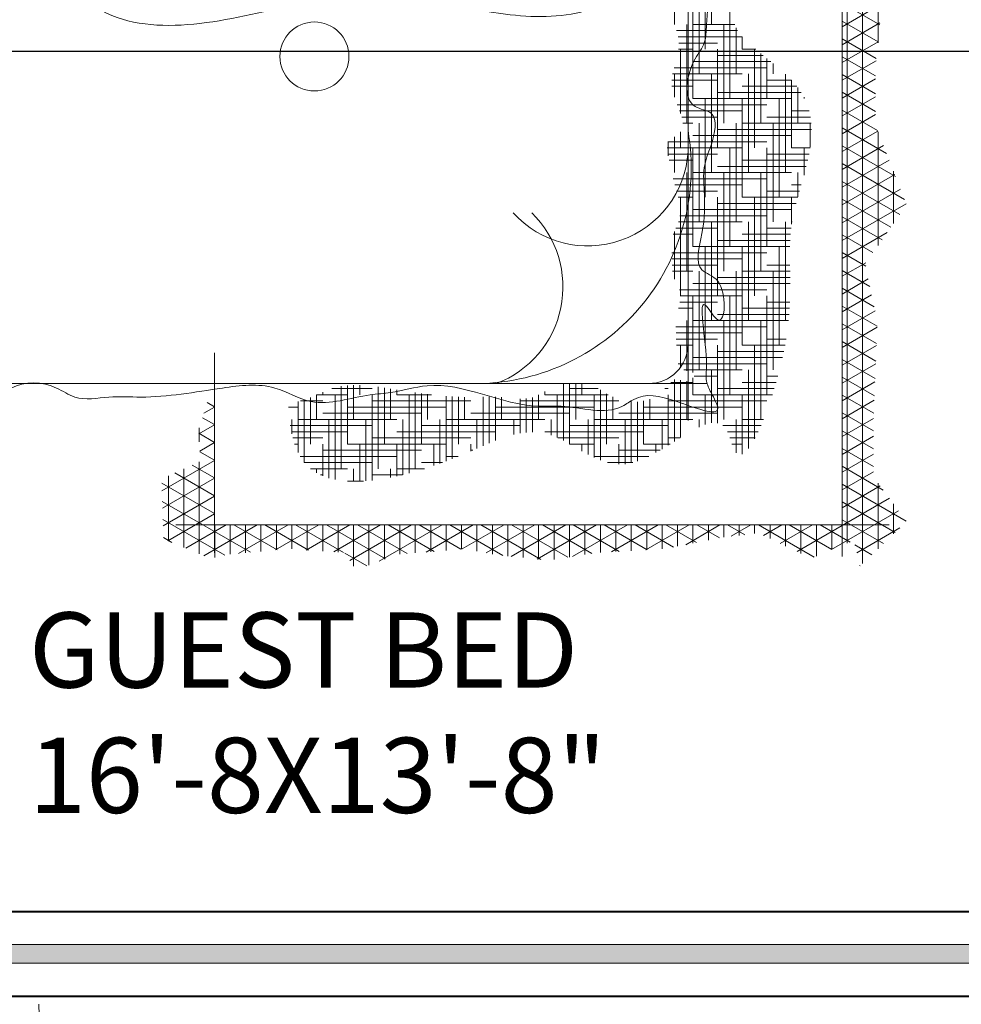
# Model space of a CAD drawing. Units: inches. Extents: x 2330 to 3943, y 1763 to 3461.
# Tile 4 of 40: x 2533 to 2634, y 2211 to 2316. Entities that reach past the tile are written whole.
import ezdxf

# ---------------------------------------------------------------- set-up
doc = ezdxf.new("R2010")
doc.units = ezdxf.units.IN
for name, color, linetype, lineweight in [('A-ANNO-DIMS', 2, 'Continuous', 18), ('A-AREA-IDEN', 7, 'Continuous', 18), ('A-FURN', 8, 'Continuous', 13), ('A-GLAZ', 4, 'Continuous', 18), ('A-WALL', 7, 'Continuous', 40), ('L-PLNT', 94, 'Continuous', 13)]:
    doc.layers.add(name, color=color, linetype=linetype, lineweight=lineweight)
doc.styles.get("Standard").update_dxf_attribs({"font": 'arial.ttf'})
doc.dimstyles.get("Standard").update_dxf_attribs({"dimtxt": 0.18, "dimasz": 0.18, "dimexe": 0.18, "dimexo": 0.0625, "dimgap": 0.09, "dimtad": 0, "dimtih": 1, "dimtoh": 1, "dimdec": 4, "dimzin": 0, "dimdsep": 46, "dimtxsty": 'Standard', "dimcen": 0.09, "dimadec": 0, "dimazin": 0, "dimtfac": 1, "dimtdec": 4, "dimtofl": 0, "dimtmove": 0, "dimatfit": 3, "dimfxl": 1, "dimtolj": 1, "dimtzin": 0, "dimarcsym": 0})

# ---------------------------------------------------------------- blocks, each defined once
blk = doc.blocks.new('A$C200C7901')
for p, q in [((2.3121, 1.6596), (2.3121, 0.0201)), ((2, 0.2957), (2, 1.2957)), ((2.0224, 0.9977), (2.0224, 1.1977)), ((2.0224, 0.9977), (2.0224, 1.1977)), ((1.9974, 0.5977), (1.9974, 0.7977)), ((1.9974, 0.5977), (1.9974, 0.7977)), ((2.0724, 0.5977), (2.0724, 0.7977)), ((2.0724, 0.5977), (2.0724, 0.7977)), ((2.1474, 0.5977), (2.1474, 0.7977)), ((2.1474, 0.5977), (2.1474, 0.7977)), ((1.9849, 0.5477), (1.9849, 0.7477)), ((1.9849, 0.5477), (1.9849, 0.7477)), ((2.0599, 0.5477), (2.0599, 0.7477)), ((2.0599, 0.5477), (2.0599, 0.7477)), ((2.1349, 0.5477), (2.1349, 0.7477)), ((2.1349, 0.5477), (2.1349, 0.7477)), ((1.0407, 0.0275), (1.0407, 0.4323)), ((0.4061, 0.3703), (2.0386, 0.3703)), ((2.4073, 0.0839), (0.9625, 0.0839))]:
    blk.add_line(p, q)
at = {"linetype": 'ByBlock'}
for p, q in [((2.3224, 0.0468), (2.3224, 1.6627)), ((2.3224, 0.0468), (2.3224, 1.6627)), ((2.3537, 0.0056), (2.3537, 1.634)), ((2.3537, 0.0056), (2.3537, 1.634)), ((2.0474, 1.0977), (2.0474, 1.2977)), ((2.0474, 1.0977), (2.0474, 1.2977)), ((2.3849, 1.0607), (2.3849, 1.3013)), ((2.3849, 1.0607), (2.3849, 1.3013)), ((1.9724, 1.0977), (1.9724, 1.2927)), ((1.9724, 1.0977), (1.9724, 1.2927)), ((2.0349, 1.0477), (2.0349, 1.2477)), ((2.0349, 1.0477), (2.0349, 1.2477)), ((2.0099, 0.9477), (2.0099, 1.1477)), ((2.0099, 0.9477), (2.0099, 1.1477)), ((2.0849, 0.9477), (2.0849, 1.1477)), ((2.0849, 0.9477), (2.0849, 1.1477)), ((2.3121, 1.1408), (2.3884, 1.0967)), ((2.3121, 1.1408), (2.3884, 1.0967)), ((2.3121, 1.0928), (2.3915, 1.1386)), ((2.3121, 1.0928), (2.3915, 1.1386)), ((1.9974, 0.8977), (1.9974, 1.0977)), ((1.9974, 0.8977), (1.9974, 1.0977)), ((2.0099, 1.0977), (2.095, 1.0977)), ((2.0099, 1.0977), (2.095, 1.0977)), ((2.0724, 0.8977), (2.0724, 1.0977)), ((2.0724, 0.8977), (2.0724, 1.0977)), ((2.3121, 1.1047), (2.3851, 1.0625)), ((2.3121, 1.1047), (2.3851, 1.0625)), ((2.3121, 1.0567), (2.3887, 1.1009)), ((2.3121, 1.0567), (2.3887, 1.1009)), ((1.9763, 1.0852), (2.1005, 1.0852)), ((1.9763, 1.0852), (2.1005, 1.0852)), ((2.0974, 0.9977), (2.0974, 1.0909)), ((2.0974, 0.9977), (2.0974, 1.0909)), ((1.9799, 1.0727), (2.1099, 1.0727)), ((1.9799, 1.0727), (2.1099, 1.0727)), ((1.9815, 1.0602), (2.0599, 1.0602)), ((1.9815, 1.0602), (2.0599, 1.0602)), ((2.1099, 1.0477), (2.1099, 1.0729)), ((2.1099, 1.0477), (2.1099, 1.0729)), ((2.3121, 1.0686), (2.3813, 1.0286)), ((2.3121, 1.0686), (2.3813, 1.0286)), ((2.3121, 1.0206), (2.3851, 1.0628)), ((2.3121, 1.0206), (2.3851, 1.0628)), ((1.981, 1.0477), (2.0099, 1.0477)), ((1.981, 1.0477), (2.0099, 1.0477)), ((1.9849, 0.9171), (1.9849, 1.0477)), ((1.9849, 0.9171), (1.9849, 1.0477)), ((2.0599, 0.8477), (2.0599, 1.0477)), ((2.0599, 0.8477), (2.0599, 1.0477)), ((2.1099, 1.0477), (2.137, 1.0477)), ((2.1099, 1.0477), (2.137, 1.0477)), ((2.1349, 0.8477), (2.1349, 1.0477)), ((2.1349, 0.8477), (2.1349, 1.0477)), ((2.1474, 0.8977), (2.1474, 1.0391)), ((2.1474, 0.8977), (2.1474, 1.0391)), ((2.0099, 1.0227), (2.1678, 1.0227)), ((2.0099, 1.0227), (2.1678, 1.0227)), ((2.0599, 1.0352), (2.1523, 1.0352)), ((2.0599, 1.0352), (2.1523, 1.0352)), ((2.1599, 0.9477), (2.1599, 1.029)), ((2.1599, 0.9477), (2.1599, 1.029)), ((2.1724, 0.9977), (2.1724, 1.0189)), ((2.1724, 0.9977), (2.1724, 1.0189)), ((2.3121, 1.0325), (2.3795, 0.9936)), ((2.3121, 1.0325), (2.3795, 0.9936)), ((2.3121, 0.9846), (2.3809, 1.0242)), ((2.3121, 0.9846), (2.3809, 1.0242)), ((1.9688, 0.9977), (2.1099, 0.9977)), ((1.9688, 0.9977), (2.1099, 0.9977)), ((1.9718, 1.0102), (2.1599, 1.0102)), ((1.9718, 1.0102), (2.1599, 1.0102)), ((1.9724, 0.9504), (1.9724, 0.9977)), ((1.9724, 0.9504), (1.9724, 0.9977)), ((2.0474, 0.7977), (2.0474, 0.9977)), ((2.0474, 0.7977), (2.0474, 0.9977)), ((2.1224, 0.7977), (2.1224, 0.9977)), ((2.1224, 0.7977), (2.1224, 0.9977)), ((1.9671, 0.9852), (2.0599, 0.9852)), ((1.9671, 0.9852), (2.0599, 0.9852)), ((2.1599, 0.9852), (2.2095, 0.9852)), ((2.1599, 0.9852), (2.2095, 0.9852)), ((2.1974, 0.7977), (2.1974, 0.9972)), ((2.1974, 0.7977), (2.1974, 0.9972)), ((2.2099, 0.8477), (2.2099, 0.9848)), ((2.2099, 0.8477), (2.2099, 0.9848)), ((2.3121, 0.9964), (2.3795, 0.9575)), ((2.3121, 0.9964), (2.3795, 0.9575)), ((2.3121, 0.9485), (2.3795, 0.9874)), ((2.3121, 0.9485), (2.3795, 0.9874)), ((1.9672, 0.9727), (2.0099, 0.9727)), ((1.9672, 0.9727), (2.0099, 0.9727)), ((2.0599, 0.9602), (2.2294, 0.9602)), ((2.0599, 0.9602), (2.2294, 0.9602)), ((2.1099, 0.9727), (2.2204, 0.9727)), ((2.1099, 0.9727), (2.2204, 0.9727)), ((2.2224, 0.8977), (2.2224, 0.9702)), ((2.2224, 0.8977), (2.2224, 0.9702)), ((2.3121, 0.9603), (2.3795, 0.9215)), ((2.3121, 0.9603), (2.3795, 0.9215)), ((2.0099, 0.9477), (2.2099, 0.9477)), ((2.0099, 0.9477), (2.2099, 0.9477)), ((2.0349, 0.7477), (2.0349, 0.9477)), ((2.0349, 0.7477), (2.0349, 0.9477)), ((2.1099, 0.7477), (2.1099, 0.9477)), ((2.1099, 0.7477), (2.1099, 0.9477)), ((2.1849, 0.7477), (2.1849, 0.9477)), ((2.1849, 0.7477), (2.1849, 0.9477)), ((2.2349, 0.9477), (2.2349, 0.9506)), ((2.2349, 0.9477), (2.2349, 0.9506)), ((2.3121, 0.9124), (2.3795, 0.9513)), ((2.3121, 0.9124), (2.3795, 0.9513)), ((1.9781, 0.9352), (2.1599, 0.9352)), ((1.9781, 0.9352), (2.1599, 0.9352)), ((1.9829, 0.9227), (2.1099, 0.9227)), ((1.9829, 0.9227), (2.1099, 0.9227)), ((2.2099, 0.9227), (2.2455, 0.9227)), ((2.2099, 0.9227), (2.2455, 0.9227)), ((2.3121, 0.9243), (2.3838, 0.8829)), ((2.3121, 0.9243), (2.3838, 0.8829)), ((1.9871, 0.9102), (2.0599, 0.9102)), ((1.9871, 0.9102), (2.0599, 0.9102)), ((2.1599, 0.9102), (2.2481, 0.9102)), ((2.1599, 0.9102), (2.2481, 0.9102)), ((2.3121, 0.8763), (2.3795, 0.9152)), ((2.3121, 0.8763), (2.3795, 0.9152)), ((1.9849, 0.8477), (1.9849, 0.88)), ((1.9849, 0.8477), (1.9849, 0.88)), ((1.9894, 0.8977), (2.0099, 0.8977)), ((1.9894, 0.8977), (2.0099, 0.8977)), ((2.0224, 0.6977), (2.0224, 0.8977)), ((2.0224, 0.6977), (2.0224, 0.8977)), ((2.0599, 0.8852), (2.2501, 0.8852)), ((2.0599, 0.8852), (2.2501, 0.8852)), ((2.0974, 0.6977), (2.0974, 0.8977)), ((2.0974, 0.6977), (2.0974, 0.8977)), ((2.1099, 0.8977), (2.2496, 0.8977)), ((2.1099, 0.8977), (2.2496, 0.8977)), ((2.1724, 0.6977), (2.1724, 0.8977)), ((2.1724, 0.6977), (2.1724, 0.8977)), ((2.2474, 0.8489), (2.2474, 0.8977)), ((2.2474, 0.8489), (2.2474, 0.8977)), ((2.3121, 0.8882), (2.4022, 0.8362)), ((2.3121, 0.8882), (2.4022, 0.8362)), ((2.3121, 0.8402), (2.3842, 0.8818)), ((2.3121, 0.8402), (2.3842, 0.8818)), ((2.3849, 0.6497), (2.3849, 0.8801)), ((2.3849, 0.6497), (2.3849, 0.8801)), ((1.9599, 0.8317), (1.9599, 0.8604)), ((1.9599, 0.8317), (1.9599, 0.8604)), ((1.9599, 0.8602), (2.1599, 0.8602)), ((1.9599, 0.8602), (2.1599, 0.8602)), ((1.9724, 0.7977), (1.9724, 0.8703)), ((1.9724, 0.7977), (1.9724, 0.8703)), ((2.0099, 0.8727), (2.2099, 0.8727)), ((2.0099, 0.8727), (2.2099, 0.8727)), ((1.9574, 0.8477), (2.1099, 0.8477)), ((1.9574, 0.8477), (2.1099, 0.8477)), ((2.0099, 0.6477), (2.0099, 0.8477)), ((2.0099, 0.6477), (2.0099, 0.8477)), ((2.0849, 0.6477), (2.0849, 0.8477)), ((2.0849, 0.6477), (2.0849, 0.8477)), ((2.1599, 0.6477), (2.1599, 0.8477)), ((2.1599, 0.6477), (2.1599, 0.8477)), ((2.2099, 0.8477), (2.2472, 0.8477)), ((2.2099, 0.8477), (2.2472, 0.8477)), ((2.2349, 0.7923), (2.2349, 0.8477)), ((2.2349, 0.7923), (2.2349, 0.8477)), ((2.3121, 0.8041), (2.3958, 0.8524)), ((2.3121, 0.8041), (2.3958, 0.8524)), ((2.3121, 0.8521), (2.4205, 0.7895)), ((2.3121, 0.8521), (2.4205, 0.7895)), ((1.9593, 0.8352), (2.0599, 0.8352)), ((1.9593, 0.8352), (2.0599, 0.8352)), ((1.9615, 0.8227), (2.0099, 0.8227)), ((1.9615, 0.8227), (2.0099, 0.8227)), ((2.1099, 0.8227), (2.2425, 0.8227)), ((2.1099, 0.8227), (2.2425, 0.8227)), ((2.1599, 0.8352), (2.2451, 0.8352)), ((2.1599, 0.8352), (2.2451, 0.8352)), ((2.3121, 0.7681), (2.4073, 0.823)), ((2.3121, 0.7681), (2.4073, 0.823)), ((2.0599, 0.8102), (2.2396, 0.8102)), ((2.0599, 0.8102), (2.2396, 0.8102)), ((2.3121, 0.816), (2.4384, 0.7431)), ((2.3121, 0.816), (2.4384, 0.7431)), ((2.4162, 0.6946), (2.4162, 0.8006)), ((2.4162, 0.6946), (2.4162, 0.8006)), ((1.9699, 0.7852), (2.1599, 0.7852)), ((1.9699, 0.7852), (2.1599, 0.7852)), ((2.0099, 0.7977), (2.2099, 0.7977)), ((2.0099, 0.7977), (2.2099, 0.7977)), ((2.2224, 0.7483), (2.2224, 0.7977)), ((2.2224, 0.7483), (2.2224, 0.7977)), ((2.3121, 0.732), (2.4189, 0.7936)), ((2.3121, 0.732), (2.4189, 0.7936)), ((2.3121, 0.7799), (2.4287, 0.7126)), ((2.3121, 0.7799), (2.4287, 0.7126)), ((1.9734, 0.7727), (2.1099, 0.7727)), ((1.9734, 0.7727), (2.1099, 0.7727)), ((1.9767, 0.7602), (2.0599, 0.7602)), ((1.9767, 0.7602), (2.0599, 0.7602)), ((2.1599, 0.7602), (2.2258, 0.7602)), ((2.1599, 0.7602), (2.2258, 0.7602)), ((2.2099, 0.7727), (2.2294, 0.7727)), ((2.2099, 0.7727), (2.2294, 0.7727)), ((2.3121, 0.6959), (2.4303, 0.7641)), ((2.3121, 0.6959), (2.4303, 0.7641)), ((1.9797, 0.7477), (2.0099, 0.7477)), ((1.9797, 0.7477), (2.0099, 0.7477)), ((2.1099, 0.7477), (2.2222, 0.7477)), ((2.1099, 0.7477), (2.2222, 0.7477)), ((2.2099, 0.6933), (2.2099, 0.7477)), ((2.2099, 0.6933), (2.2099, 0.7477)), ((2.3121, 0.7438), (2.4108, 0.6869)), ((2.3121, 0.7438), (2.4108, 0.6869)), ((2.0099, 0.7227), (2.2099, 0.7227)), ((2.0099, 0.7227), (2.2099, 0.7227)), ((2.0599, 0.7352), (2.2188, 0.7352)), ((2.0599, 0.7352), (2.2188, 0.7352)), ((2.3121, 0.6598), (2.4417, 0.7346)), ((2.3121, 0.6598), (2.4417, 0.7346)), ((1.9831, 0.7102), (2.1599, 0.7102)), ((1.9831, 0.7102), (2.1599, 0.7102)), ((2.3121, 0.7078), (2.3929, 0.6611)), ((2.3121, 0.7078), (2.3929, 0.6611)), ((1.9724, 0.5818), (1.9724, 0.6786)), ((1.9724, 0.5818), (1.9724, 0.6786)), ((1.9753, 0.6852), (2.0599, 0.6852)), ((1.9753, 0.6852), (2.0599, 0.6852)), ((1.9804, 0.6977), (2.1099, 0.6977)), ((1.9804, 0.6977), (2.1099, 0.6977)), ((2.0474, 0.4977), (2.0474, 0.6977)), ((2.0474, 0.4977), (2.0474, 0.6977)), ((2.1224, 0.4977), (2.1224, 0.6977)), ((2.1224, 0.4977), (2.1224, 0.6977)), ((2.1599, 0.6852), (2.2088, 0.6852)), ((2.1599, 0.6852), (2.2088, 0.6852)), ((2.1974, 0.4977), (2.1974, 0.6977)), ((2.1974, 0.4977), (2.1974, 0.6977)), ((2.2099, 0.6977), (2.2106, 0.6977)), ((2.2099, 0.6977), (2.2106, 0.6977)), ((1.97, 0.6727), (2.0099, 0.6727)), ((1.97, 0.6727), (2.0099, 0.6727)), ((2.0599, 0.6602), (2.2067, 0.6602)), ((2.0599, 0.6602), (2.2067, 0.6602)), ((2.1099, 0.6727), (2.2075, 0.6727)), ((2.1099, 0.6727), (2.2075, 0.6727)), ((2.3121, 0.6237), (2.4036, 0.6765)), ((2.3121, 0.6237), (2.4036, 0.6765)), ((2.3121, 0.6717), (2.3744, 0.6357)), ((2.3121, 0.6717), (2.3744, 0.6357)), ((2.0099, 0.6477), (2.2062, 0.6477)), ((2.0099, 0.6477), (2.2062, 0.6477)), ((2.0349, 0.4477), (2.0349, 0.6477)), ((2.0349, 0.4477), (2.0349, 0.6477)), ((2.1099, 0.4477), (2.1099, 0.6477)), ((2.1099, 0.4477), (2.1099, 0.6477)), ((2.1849, 0.4477), (2.1849, 0.6477)), ((2.1849, 0.4477), (2.1849, 0.6477)), ((1.9673, 0.6352), (2.1599, 0.6352)), ((1.9673, 0.6352), (2.1599, 0.6352)), ((1.9678, 0.6227), (2.1099, 0.6227)), ((1.9678, 0.6227), (2.1099, 0.6227)), ((2.3121, 0.6356), (2.3598, 0.6081)), ((2.3121, 0.6356), (2.3598, 0.6081)), ((1.9679, 0.6102), (2.0599, 0.6102)), ((1.9679, 0.6102), (2.0599, 0.6102)), ((2.1599, 0.6102), (2.2064, 0.6102)), ((2.1599, 0.6102), (2.2064, 0.6102)), ((2.3121, 0.5876), (2.3598, 0.6151)), ((2.3121, 0.5876), (2.3598, 0.6151)), ((2.3121, 0.5995), (2.3682, 0.5671)), ((2.3121, 0.5995), (2.3682, 0.5671)), ((1.9685, 0.5977), (2.0099, 0.5977)), ((1.9685, 0.5977), (2.0099, 0.5977)), ((2.0224, 0.3977), (2.0224, 0.5977)), ((2.0224, 0.3977), (2.0224, 0.5977)), ((2.0599, 0.5852), (2.2069, 0.5852)), ((2.0599, 0.5852), (2.2069, 0.5852)), ((2.0974, 0.3977), (2.0974, 0.5977)), ((2.0974, 0.3977), (2.0974, 0.5977)), ((2.1099, 0.5977), (2.2066, 0.5977)), ((2.1099, 0.5977), (2.2066, 0.5977)), ((2.1724, 0.3977), (2.1724, 0.5977)), ((2.1724, 0.3977), (2.1724, 0.5977)), ((2.3121, 0.5515), (2.365, 0.5821)), ((2.3121, 0.5515), (2.365, 0.5821)), ((1.9827, 0.5602), (2.1599, 0.5602)), ((1.9827, 0.5602), (2.1599, 0.5602)), ((2.0099, 0.5727), (2.207, 0.5727)), ((2.0099, 0.5727), (2.207, 0.5727)), ((2.3121, 0.5634), (2.3771, 0.5259)), ((2.3121, 0.5634), (2.3771, 0.5259)), ((1.9842, 0.5477), (2.1099, 0.5477)), ((1.9842, 0.5477), (2.1099, 0.5477)), ((2.0099, 0.3923), (2.0099, 0.5477)), ((2.0099, 0.3923), (2.0099, 0.5477)), ((2.0849, 0.3477), (2.0849, 0.5477)), ((2.0849, 0.3477), (2.0849, 0.5477)), ((2.1599, 0.3477), (2.1599, 0.5477)), ((2.1599, 0.3477), (2.1599, 0.5477)), ((2.3121, 0.5155), (2.3719, 0.55)), ((2.3121, 0.5155), (2.3719, 0.55)), ((1.9807, 0.5227), (2.0099, 0.5227)), ((1.9807, 0.5227), (2.0099, 0.5227)), ((1.9831, 0.5352), (2.0599, 0.5352)), ((1.9831, 0.5352), (2.0599, 0.5352)), ((2.1099, 0.5227), (2.2058, 0.5227)), ((2.1099, 0.5227), (2.2058, 0.5227)), ((2.1599, 0.5352), (2.2065, 0.5352)), ((2.1599, 0.5352), (2.2065, 0.5352)), ((2.3121, 0.5273), (2.383, 0.4864)), ((2.3121, 0.5273), (2.383, 0.4864)), ((2.0599, 0.5102), (2.2049, 0.5102)), ((2.0599, 0.5102), (2.2049, 0.5102)), ((2.3121, 0.4794), (2.3788, 0.5179)), ((2.3121, 0.4794), (2.3788, 0.5179)), ((1.9755, 0.4852), (2.1599, 0.4852)), ((1.9755, 0.4852), (2.1599, 0.4852)), ((1.9974, 0.3957), (1.9974, 0.4977)), ((1.9974, 0.3957), (1.9974, 0.4977)), ((2.0099, 0.4977), (2.2038, 0.4977)), ((2.0099, 0.4977), (2.2038, 0.4977)), ((2.0724, 0.2977), (2.0724, 0.4977)), ((2.0724, 0.2977), (2.0724, 0.4977)), ((2.1474, 0.2977), (2.1474, 0.4977)), ((2.1474, 0.2977), (2.1474, 0.4977)), ((2.3121, 0.4912), (2.3817, 0.4511)), ((2.3121, 0.4912), (2.3817, 0.4511)), ((2.3121, 0.4433), (2.383, 0.4842)), ((2.3121, 0.4433), (2.383, 0.4842)), ((1.9757, 0.4727), (2.1099, 0.4727)), ((1.9757, 0.4727), (2.1099, 0.4727)), ((1.9762, 0.4602), (2.0599, 0.4602)), ((1.9762, 0.4602), (2.0599, 0.4602)), ((2.1599, 0.4602), (2.1987, 0.4602)), ((2.1599, 0.4602), (2.1987, 0.4602)), ((1.9768, 0.4477), (2.0099, 0.4477)), ((1.9768, 0.4477), (2.0099, 0.4477)), ((1.9849, 0.402), (1.9849, 0.4477)), ((1.9849, 0.402), (1.9849, 0.4477)), ((2.0599, 0.2903), (2.0599, 0.4477)), ((2.0599, 0.2903), (2.0599, 0.4477)), ((2.1099, 0.4477), (2.1965, 0.4477)), ((2.1099, 0.4477), (2.1965, 0.4477)), ((2.1349, 0.2582), (2.1349, 0.4477)), ((2.1349, 0.2582), (2.1349, 0.4477)), ((2.3121, 0.4552), (2.3803, 0.4158)), ((2.3121, 0.4552), (2.3803, 0.4158)), ((2.3121, 0.4072), (2.3815, 0.4473)), ((2.3121, 0.4072), (2.3815, 0.4473)), ((2.0099, 0.4227), (2.1913, 0.4227)), ((2.0099, 0.4227), (2.1913, 0.4227)), ((2.0599, 0.4352), (2.194, 0.4352)), ((2.0599, 0.4352), (2.194, 0.4352)), ((2.3121, 0.4191), (2.3789, 0.3805)), ((2.3121, 0.4191), (2.3789, 0.3805)), ((1.9797, 0.4102), (2.1599, 0.4102)), ((1.9797, 0.4102), (2.1599, 0.4102)), ((2.3121, 0.3711), (2.3801, 0.4103)), ((2.3121, 0.3711), (2.3801, 0.4103)), ((1.9915, 0.3977), (2.1099, 0.3977)), ((1.9915, 0.3977), (2.1099, 0.3977)), ((2.0099, 0.3477), (2.0099, 0.382)), ((2.0099, 0.3477), (2.0099, 0.382)), ((2.0127, 0.3852), (2.0599, 0.3852)), ((2.0127, 0.3852), (2.0599, 0.3852)), ((2.0474, 0.2905), (2.0474, 0.3977)), ((2.0474, 0.2905), (2.0474, 0.3977)), ((2.1224, 0.2385), (2.1224, 0.3977)), ((2.1224, 0.2385), (2.1224, 0.3977)), ((2.1599, 0.3852), (2.1819, 0.3852)), ((2.1599, 0.3852), (2.1819, 0.3852)), ((2.3121, 0.383), (2.3775, 0.3452)), ((2.3121, 0.383), (2.3775, 0.3452)), ((1.2785, 0.3602), (1.3599, 0.3602)), ((1.2785, 0.3602), (1.3599, 0.3602)), ((1.2974, 0.1977), (1.2974, 0.3647)), ((1.2974, 0.1977), (1.2974, 0.3647)), ((1.3099, 0.2477), (1.3099, 0.3663)), ((1.3099, 0.2477), (1.3099, 0.3663)), ((1.3224, 0.2977), (1.3224, 0.3669)), ((1.3224, 0.2977), (1.3224, 0.3669)), ((1.3349, 0.3477), (1.3349, 0.3668)), ((1.3349, 0.3477), (1.3349, 0.3668)), ((1.3724, 0.1977), (1.3724, 0.3634)), ((1.3724, 0.1977), (1.3724, 0.3634)), ((1.3849, 0.2477), (1.3849, 0.3616)), ((1.3849, 0.2477), (1.3849, 0.3616)), ((1.3974, 0.2977), (1.3974, 0.3597)), ((1.3974, 0.2977), (1.3974, 0.3597)), ((1.7474, 0.2546), (1.7474, 0.3689)), ((1.7474, 0.2546), (1.7474, 0.3689)), ((1.7599, 0.2477), (1.7599, 0.3703)), ((1.7599, 0.2477), (1.7599, 0.3703)), ((1.7599, 0.3602), (1.8177, 0.3602)), ((1.7599, 0.3602), (1.8177, 0.3602)), ((1.7724, 0.2977), (1.7724, 0.3703)), ((1.7724, 0.2977), (1.7724, 0.3703)), ((1.7849, 0.3477), (1.7849, 0.3703)), ((1.7849, 0.3477), (1.7849, 0.3703)), ((1.9532, 0.3602), (1.9599, 0.3602)), ((1.9532, 0.3602), (1.9599, 0.3602)), ((1.9648, 0.3727), (2.0099, 0.3727)), ((1.9648, 0.3727), (2.0099, 0.3727)), ((1.9724, 0.253), (1.9724, 0.3785)), ((1.9724, 0.253), (1.9724, 0.3785)), ((1.9849, 0.2609), (1.9849, 0.3774)), ((1.9849, 0.2609), (1.9849, 0.3774)), ((1.9974, 0.2977), (1.9974, 0.3753)), ((1.9974, 0.2977), (1.9974, 0.3753)), ((2.0599, 0.3602), (2.1747, 0.3602)), ((2.0599, 0.3602), (2.1747, 0.3602)), ((2.1099, 0.3727), (2.1784, 0.3727)), ((2.1099, 0.3727), (2.1784, 0.3727)), ((2.3121, 0.335), (2.3786, 0.3734)), ((2.3121, 0.335), (2.3786, 0.3734)), ((1.2349, 0.2477), (1.2349, 0.3422)), ((1.2349, 0.2477), (1.2349, 0.3422)), ((1.2474, 0.2977), (1.2474, 0.3476)), ((1.2474, 0.2977), (1.2474, 0.3476)), ((1.2475, 0.3477), (1.3099, 0.3477)), ((1.2475, 0.3477), (1.3099, 0.3477)), ((1.2599, 0.3477), (1.2599, 0.3531)), ((1.2599, 0.3477), (1.2599, 0.3531)), ((1.2849, 0.1758), (1.2849, 0.3477)), ((1.2849, 0.1758), (1.2849, 0.3477)), ((1.3599, 0.1741), (1.3599, 0.3477)), ((1.3599, 0.1741), (1.3599, 0.3477)), ((1.4099, 0.3477), (1.4099, 0.3578)), ((1.4099, 0.3477), (1.4099, 0.3578)), ((1.4099, 0.3477), (1.4806, 0.3477)), ((1.4099, 0.3477), (1.4806, 0.3477)), ((1.4349, 0.1886), (1.4349, 0.3477)), ((1.4349, 0.1886), (1.4349, 0.3477)), ((1.4474, 0.1977), (1.4474, 0.3521)), ((1.4474, 0.1977), (1.4474, 0.3521)), ((1.4599, 0.2477), (1.4599, 0.3504)), ((1.4599, 0.2477), (1.4599, 0.3504)), ((1.4724, 0.2977), (1.4724, 0.3487)), ((1.4724, 0.2977), (1.4724, 0.3487)), ((1.5099, 0.2129), (1.5099, 0.3447)), ((1.5099, 0.2129), (1.5099, 0.3447)), ((1.5224, 0.2177), (1.5224, 0.3438)), ((1.5224, 0.2177), (1.5224, 0.3438)), ((1.5349, 0.2477), (1.5349, 0.3431)), ((1.5349, 0.2477), (1.5349, 0.3431)), ((1.5474, 0.2977), (1.5474, 0.3428)), ((1.5474, 0.2977), (1.5474, 0.3428)), ((1.5849, 0.2443), (1.5849, 0.3434)), ((1.5849, 0.2443), (1.5849, 0.3434)), ((1.5974, 0.2496), (1.5974, 0.3435)), ((1.5974, 0.2496), (1.5974, 0.3435)), ((1.6099, 0.2546), (1.6099, 0.3432)), ((1.6099, 0.2546), (1.6099, 0.3432)), ((1.6224, 0.2977), (1.6224, 0.3424)), ((1.6224, 0.2977), (1.6224, 0.3424)), ((1.6599, 0.2695), (1.6599, 0.3394)), ((1.6599, 0.2695), (1.6599, 0.3394)), ((1.6724, 0.2713), (1.6724, 0.3398)), ((1.6724, 0.2713), (1.6724, 0.3398)), ((1.6849, 0.272), (1.6849, 0.3422)), ((1.6849, 0.272), (1.6849, 0.3422)), ((1.6974, 0.2977), (1.6974, 0.3472)), ((1.6974, 0.2977), (1.6974, 0.3472)), ((1.7099, 0.3477), (1.7099, 0.3539)), ((1.7099, 0.3477), (1.7099, 0.3539)), ((1.7099, 0.3477), (1.8383, 0.3477)), ((1.7099, 0.3477), (1.8383, 0.3477)), ((1.7349, 0.2607), (1.7349, 0.3477)), ((1.7349, 0.2607), (1.7349, 0.3477)), ((1.8099, 0.2201), (1.8099, 0.3477)), ((1.8099, 0.2201), (1.8099, 0.3477)), ((1.8224, 0.2148), (1.8224, 0.3575)), ((1.8224, 0.2148), (1.8224, 0.3575)), ((1.8349, 0.2477), (1.8349, 0.3497)), ((1.8349, 0.2477), (1.8349, 0.3497)), ((1.8474, 0.2977), (1.8474, 0.3432)), ((1.8474, 0.2977), (1.8474, 0.3432)), ((1.9599, 0.2452), (1.9599, 0.3477)), ((1.9599, 0.2452), (1.9599, 0.3477)), ((2.0099, 0.3477), (2.1708, 0.3477)), ((2.0099, 0.3477), (2.1708, 0.3477)), ((2.0349, 0.2874), (2.0349, 0.3477)), ((2.0349, 0.2874), (2.0349, 0.3477)), ((2.1099, 0.2274), (2.1099, 0.3477)), ((2.1099, 0.2274), (2.1099, 0.3477)), ((2.3121, 0.3469), (2.3761, 0.31)), ((2.3121, 0.3469), (2.3761, 0.31)), ((1.0194, 0.3103), (1.0407, 0.3227)), ((1.0194, 0.3103), (1.0407, 0.3227)), ((1.0261, 0.3316), (1.0407, 0.3232)), ((1.0261, 0.3316), (1.0407, 0.3232)), ((1.1904, 0.3227), (1.2099, 0.3227)), ((1.1904, 0.3227), (1.2099, 0.3227)), ((1.2099, 0.2308), (1.2099, 0.334)), ((1.2099, 0.2308), (1.2099, 0.334)), ((1.2148, 0.3352), (1.2599, 0.3352)), ((1.2148, 0.3352), (1.2599, 0.3352)), ((1.2224, 0.2106), (1.2224, 0.3375)), ((1.2224, 0.2106), (1.2224, 0.3375)), ((1.3099, 0.3227), (1.5099, 0.3227)), ((1.3099, 0.3227), (1.5099, 0.3227)), ((1.3599, 0.3352), (1.5599, 0.3352)), ((1.3599, 0.3352), (1.5599, 0.3352)), ((1.6099, 0.3227), (1.8099, 0.3227)), ((1.6099, 0.3227), (1.8099, 0.3227)), ((1.6599, 0.3352), (1.8599, 0.3352)), ((1.6599, 0.3352), (1.8599, 0.3352)), ((1.8849, 0.2093), (1.8849, 0.3337)), ((1.8849, 0.2093), (1.8849, 0.3337)), ((1.8974, 0.2129), (1.8974, 0.3335)), ((1.8974, 0.2129), (1.8974, 0.3335)), ((1.9099, 0.2477), (1.9099, 0.3349)), ((1.9099, 0.2477), (1.9099, 0.3349)), ((1.9099, 0.3227), (2.1099, 0.3227)), ((1.9099, 0.3227), (2.1099, 0.3227)), ((1.9224, 0.2977), (1.9224, 0.3385)), ((1.9224, 0.2977), (1.9224, 0.3385)), ((1.9599, 0.3352), (2.1599, 0.3352)), ((1.9599, 0.3352), (2.1599, 0.3352)), ((2.3121, 0.299), (2.3772, 0.3365)), ((2.3121, 0.299), (2.3772, 0.3365)), ((1.0164, 0.3011), (1.0407, 0.2871)), ((1.0164, 0.3011), (1.0407, 0.2871)), ((1.2599, 0.3102), (1.4599, 0.3102)), ((1.2599, 0.3102), (1.4599, 0.3102)), ((1.5599, 0.3102), (1.7599, 0.3102)), ((1.5599, 0.3102), (1.7599, 0.3102)), ((1.8599, 0.3102), (2.0599, 0.3102)), ((1.8599, 0.3102), (2.0599, 0.3102)), ((2.3121, 0.3108), (2.3755, 0.2742)), ((2.3121, 0.3108), (2.3755, 0.2742)), ((2.3121, 0.2629), (2.3757, 0.2996)), ((2.3121, 0.2629), (2.3757, 0.2996)), ((1.0089, 0.2682), (1.0407, 0.2866)), ((1.0089, 0.2682), (1.0407, 0.2866)), ((1.0099, 0.2521), (1.0099, 0.2804)), ((1.0099, 0.2521), (1.0099, 0.2804)), ((1.1943, 0.2852), (1.3599, 0.2852)), ((1.1943, 0.2852), (1.3599, 0.2852)), ((1.1974, 0.2683), (1.1974, 0.2977)), ((1.1974, 0.2683), (1.1974, 0.2977)), ((1.2099, 0.2977), (1.4099, 0.2977)), ((1.2099, 0.2977), (1.4099, 0.2977)), ((1.2724, 0.1788), (1.2724, 0.2977)), ((1.2724, 0.1788), (1.2724, 0.2977)), ((1.3474, 0.173), (1.3474, 0.2977)), ((1.3474, 0.173), (1.3474, 0.2977)), ((1.4224, 0.1854), (1.4224, 0.2977)), ((1.4224, 0.1854), (1.4224, 0.2977)), ((1.4599, 0.2852), (1.6599, 0.2852)), ((1.4599, 0.2852), (1.6599, 0.2852)), ((1.4974, 0.2083), (1.4974, 0.2977)), ((1.4974, 0.2083), (1.4974, 0.2977)), ((1.5099, 0.2977), (1.7099, 0.2977)), ((1.5099, 0.2977), (1.7099, 0.2977)), ((1.5724, 0.2389), (1.5724, 0.2977)), ((1.5724, 0.2389), (1.5724, 0.2977)), ((1.6474, 0.2668), (1.6474, 0.2977)), ((1.6474, 0.2668), (1.6474, 0.2977)), ((1.7224, 0.2658), (1.7224, 0.2977)), ((1.7224, 0.2658), (1.7224, 0.2977)), ((1.7599, 0.2852), (1.9599, 0.2852)), ((1.7599, 0.2852), (1.9599, 0.2852)), ((1.7974, 0.2263), (1.7974, 0.2977)), ((1.7974, 0.2263), (1.7974, 0.2977)), ((1.8099, 0.2977), (2.0099, 0.2977)), ((1.8099, 0.2977), (2.0099, 0.2977)), ((1.8724, 0.2072), (1.8724, 0.2977)), ((1.8724, 0.2072), (1.8724, 0.2977)), ((1.9474, 0.2376), (1.9474, 0.2977)), ((1.9474, 0.2376), (1.9474, 0.2977)), ((2.0224, 0.2822), (2.0224, 0.2977)), ((2.0224, 0.2822), (2.0224, 0.2977)), ((2.0708, 0.2852), (2.1478, 0.2852)), ((2.0708, 0.2852), (2.1478, 0.2852)), ((2.0974, 0.2299), (2.0974, 0.2977)), ((2.0974, 0.2299), (2.0974, 0.2977)), ((2.1099, 0.2977), (2.153, 0.2977)), ((2.1099, 0.2977), (2.153, 0.2977)), ((1.0088, 0.2694), (1.0407, 0.251)), ((1.0088, 0.2694), (1.0407, 0.251)), ((1.1965, 0.2727), (1.3099, 0.2727)), ((1.1965, 0.2727), (1.3099, 0.2727)), ((1.1994, 0.2602), (1.2599, 0.2602)), ((1.1994, 0.2602), (1.2599, 0.2602)), ((1.3599, 0.2602), (1.5599, 0.2602)), ((1.3599, 0.2602), (1.5599, 0.2602)), ((1.4099, 0.2727), (1.6099, 0.2727)), ((1.4099, 0.2727), (1.6099, 0.2727)), ((1.7099, 0.2727), (1.9099, 0.2727)), ((1.7099, 0.2727), (1.9099, 0.2727)), ((1.7361, 0.2602), (1.8599, 0.2602)), ((1.7361, 0.2602), (1.8599, 0.2602)), ((1.9599, 0.2602), (1.9838, 0.2602)), ((1.9599, 0.2602), (1.9838, 0.2602)), ((2.08, 0.2727), (2.1422, 0.2727)), ((2.08, 0.2727), (2.1422, 0.2727)), ((2.0848, 0.2602), (2.1359, 0.2602)), ((2.0848, 0.2602), (2.1359, 0.2602)), ((2.3121, 0.2747), (2.3755, 0.2381)), ((2.3121, 0.2747), (2.3755, 0.2381)), ((2.3121, 0.2268), (2.3755, 0.2634)), ((2.3121, 0.2268), (2.3755, 0.2634)), ((1.0111, 0.2334), (1.0407, 0.2505)), ((1.0111, 0.2334), (1.0407, 0.2505)), ((1.2031, 0.2477), (1.2099, 0.2477)), ((1.2031, 0.2477), (1.2099, 0.2477)), ((1.2599, 0.1831), (1.2599, 0.2477)), ((1.2599, 0.1831), (1.2599, 0.2477)), ((1.3099, 0.2477), (1.5099, 0.2477)), ((1.3099, 0.2477), (1.5099, 0.2477)), ((1.3349, 0.1723), (1.3349, 0.2477)), ((1.3349, 0.1723), (1.3349, 0.2477)), ((1.4099, 0.1825), (1.4099, 0.2477)), ((1.4099, 0.1825), (1.4099, 0.2477)), ((1.4849, 0.2039), (1.4849, 0.2477)), ((1.4849, 0.2039), (1.4849, 0.2477)), ((1.5599, 0.2335), (1.5599, 0.2477)), ((1.5599, 0.2335), (1.5599, 0.2477)), ((1.7599, 0.2477), (1.8099, 0.2477)), ((1.7599, 0.2477), (1.8099, 0.2477)), ((1.7849, 0.2332), (1.7849, 0.2477)), ((1.7849, 0.2332), (1.7849, 0.2477)), ((1.8599, 0.2068), (1.8599, 0.2477)), ((1.8599, 0.2068), (1.8599, 0.2477)), ((1.9099, 0.2477), (1.9639, 0.2477)), ((1.9099, 0.2477), (1.9639, 0.2477)), ((1.9349, 0.2304), (1.9349, 0.2477)), ((1.9349, 0.2304), (1.9349, 0.2477)), ((2.0888, 0.2477), (2.1099, 0.2477)), ((2.0888, 0.2477), (2.1099, 0.2477)), ((1.0112, 0.232), (1.0407, 0.215)), ((1.0112, 0.232), (1.0407, 0.215)), ((1.2142, 0.2227), (1.4099, 0.2227)), ((1.2142, 0.2227), (1.4099, 0.2227)), ((1.2599, 0.2352), (1.4599, 0.2352)), ((1.2599, 0.2352), (1.4599, 0.2352)), ((1.5099, 0.2227), (1.5346, 0.2227)), ((1.5099, 0.2227), (1.5346, 0.2227)), ((1.5599, 0.2352), (1.5638, 0.2352)), ((1.5599, 0.2352), (1.5638, 0.2352)), ((1.8099, 0.2227), (1.9203, 0.2227)), ((1.8099, 0.2227), (1.9203, 0.2227)), ((1.8599, 0.2352), (1.9433, 0.2352)), ((1.8599, 0.2352), (1.9433, 0.2352)), ((2.3121, 0.2387), (2.3755, 0.202)), ((2.3121, 0.2387), (2.3755, 0.202)), ((2.3121, 0.1907), (2.3755, 0.2273)), ((2.3121, 0.1907), (2.3755, 0.2273)), ((0.9344, 0.153), (1.0407, 0.2144)), ((0.9344, 0.153), (1.0407, 0.2144)), ((0.9953, 0.2051), (1.0407, 0.1789)), ((0.9953, 0.2051), (1.0407, 0.1789)), ((1.0099, 0.0251), (1.0099, 0.2117)), ((1.0099, 0.0251), (1.0099, 0.2117)), ((1.2227, 0.2102), (1.3599, 0.2102)), ((1.2227, 0.2102), (1.3599, 0.2102)), ((1.4599, 0.2102), (1.5027, 0.2102)), ((1.4599, 0.2102), (1.5027, 0.2102)), ((1.8368, 0.2102), (1.8884, 0.2102)), ((1.8368, 0.2102), (1.8884, 0.2102)), ((2.3121, 0.2026), (2.3953, 0.1545)), ((2.3121, 0.2026), (2.3953, 0.1545)), ((0.9474, 0.0512), (0.9474, 0.1835)), ((0.9474, 0.0512), (0.9474, 0.1835)), ((0.9602, 0.1893), (1.0407, 0.1428)), ((0.9602, 0.1893), (1.0407, 0.1428)), ((0.9787, 0.0381), (0.9787, 0.1976)), ((0.9787, 0.0381), (0.9787, 0.1976)), ((1.2351, 0.1977), (1.3099, 0.1977)), ((1.2351, 0.1977), (1.3099, 0.1977)), ((1.2474, 0.1892), (1.2474, 0.1977)), ((1.2474, 0.1892), (1.2474, 0.1977)), ((1.2552, 0.1852), (1.2599, 0.1852)), ((1.2552, 0.1852), (1.2599, 0.1852)), ((1.3224, 0.1722), (1.3224, 0.1977)), ((1.3224, 0.1722), (1.3224, 0.1977)), ((1.3599, 0.1852), (1.4215, 0.1852)), ((1.3599, 0.1852), (1.4215, 0.1852)), ((1.3974, 0.1799), (1.3974, 0.1977)), ((1.3974, 0.1799), (1.3974, 0.1977)), ((1.4099, 0.1977), (1.4662, 0.1977)), ((1.4099, 0.1977), (1.4662, 0.1977)), ((2.3121, 0.1546), (2.3755, 0.1912)), ((2.3121, 0.1546), (2.3755, 0.1912)), ((0.9339, 0.1684), (1.0407, 0.1067)), ((0.9339, 0.1684), (1.0407, 0.1067)), ((0.9355, 0.1176), (1.0407, 0.1783)), ((0.9355, 0.1176), (1.0407, 0.1783)), ((1.3099, 0.1727), (1.3428, 0.1727)), ((1.3099, 0.1727), (1.3428, 0.1727)), ((2.3121, 0.1665), (2.4419, 0.0916)), ((2.3121, 0.1665), (2.4419, 0.0916)), ((2.3121, 0.1185), (2.3891, 0.163)), ((2.3121, 0.1185), (2.3891, 0.163)), ((2.3849, 0.0355), (2.3849, 0.1686)), ((2.3849, 0.0355), (2.3849, 0.1686)), ((0.9366, 0.0822), (1.0407, 0.1422)), ((0.9366, 0.0822), (1.0407, 0.1422)), ((0.935, 0.1316), (1.114, 0.0283)), ((0.935, 0.1316), (1.114, 0.0283)), ((2.2208, 0.0297), (2.4078, 0.1377)), ((2.2208, 0.0297), (2.4078, 0.1377)), ((2.3121, 0.1304), (2.4193, 0.0685)), ((2.3121, 0.1304), (2.4193, 0.0685)), ((2.4162, 0.0655), (2.4162, 0.1264)), ((2.4162, 0.0655), (2.4162, 0.1264)), ((0.9463, 0.0516), (1.0407, 0.1061)), ((0.9463, 0.0516), (1.0407, 0.1061)), ((2.2903, 0.0337), (2.4265, 0.1124)), ((2.2903, 0.0337), (2.4265, 0.1124)), ((0.9362, 0.0948), (1.0616, 0.0225)), ((0.9362, 0.0948), (1.0616, 0.0225)), ((0.9826, 0.0365), (1.0647, 0.0839)), ((0.9826, 0.0365), (1.0647, 0.0839)), ((1.0189, 0.0214), (1.1272, 0.0839)), ((1.0189, 0.0214), (1.1272, 0.0839)), ((1.0412, 0.0179), (1.0412, 0.0839)), ((1.0412, 0.0179), (1.0412, 0.0839)), ((1.0724, 0.0243), (1.0724, 0.0839)), ((1.0724, 0.0243), (1.0724, 0.0839)), ((1.0801, 0.0839), (1.1675, 0.0335)), ((1.0801, 0.0839), (1.1675, 0.0335)), ((1.0891, 0.0259), (1.1897, 0.0839)), ((1.0891, 0.0259), (1.1897, 0.0839)), ((1.1037, 0.0273), (1.1037, 0.0839)), ((1.1037, 0.0273), (1.1037, 0.0839)), ((1.1349, 0.0303), (1.1349, 0.0839)), ((1.1349, 0.0303), (1.1349, 0.0839)), ((1.1426, 0.0839), (1.2313, 0.0327)), ((1.1426, 0.0839), (1.2313, 0.0327)), ((1.1642, 0.0331), (1.2522, 0.0839)), ((1.1642, 0.0331), (1.2522, 0.0839)), ((1.1662, 0.0333), (1.1662, 0.0839)), ((1.1662, 0.0333), (1.1662, 0.0839)), ((1.1974, 0.0351), (1.1974, 0.0839)), ((1.1974, 0.0351), (1.1974, 0.0839)), ((1.2051, 0.0839), (1.3023, 0.0278)), ((1.2051, 0.0839), (1.3023, 0.0278)), ((1.2266, 0.033), (1.3147, 0.0839)), ((1.2266, 0.033), (1.3147, 0.0839)), ((1.2287, 0.0329), (1.2287, 0.0839)), ((1.2287, 0.0329), (1.2287, 0.0839)), ((1.2599, 0.0308), (1.2599, 0.0839)), ((1.2599, 0.0308), (1.2599, 0.0839)), ((1.2676, 0.0839), (1.3871, 0.015)), ((1.2676, 0.0839), (1.3871, 0.015)), ((1.2824, 0.0292), (1.3772, 0.0839)), ((1.2824, 0.0292), (1.3772, 0.0839)), ((1.2912, 0.0286), (1.2912, 0.0839)), ((1.2912, 0.0286), (1.2912, 0.0839)), ((1.3146, 0.0117), (1.4397, 0.0839)), ((1.3146, 0.0117), (1.4397, 0.0839)), ((1.3224, 0), (1.3224, 0.0839)), ((1.3224, 0), (1.3224, 0.0839)), ((1.3301, 0.0839), (1.4312, 0.0256)), ((1.3301, 0.0839), (1.4312, 0.0256)), ((1.3537, 0.0022), (1.3537, 0.0839)), ((1.3537, 0.0022), (1.3537, 0.0839)), ((1.3743, 0.0101), (1.5022, 0.0839)), ((1.3743, 0.0101), (1.5022, 0.0839)), ((1.3849, 0.0141), (1.3849, 0.0839)), ((1.3849, 0.0141), (1.3849, 0.0839)), ((1.3926, 0.0839), (1.4856, 0.0302)), ((1.3926, 0.0839), (1.4856, 0.0302)), ((1.4162, 0.0243), (1.4162, 0.0839)), ((1.4162, 0.0243), (1.4162, 0.0839)), ((1.4474, 0.027), (1.4474, 0.0839)), ((1.4474, 0.027), (1.4474, 0.0839)), ((1.4551, 0.0839), (1.54, 0.0349)), ((1.4551, 0.0839), (1.54, 0.0349)), ((1.4693, 0.0288), (1.5647, 0.0839)), ((1.4693, 0.0288), (1.5647, 0.0839)), ((1.4787, 0.0296), (1.4787, 0.0839)), ((1.4787, 0.0296), (1.4787, 0.0839)), ((1.5099, 0.0323), (1.5099, 0.0839)), ((1.5099, 0.0323), (1.5099, 0.0839)), ((1.5176, 0.0839), (1.6251, 0.0219)), ((1.5176, 0.0839), (1.6251, 0.0219)), ((1.5412, 0.035), (1.5412, 0.0839)), ((1.5412, 0.035), (1.5412, 0.0839)), ((1.5427, 0.0351), (1.6272, 0.0839)), ((1.5427, 0.0351), (1.6272, 0.0839)), ((1.5724, 0.0308), (1.5724, 0.0839)), ((1.5724, 0.0308), (1.5724, 0.0839)), ((1.5801, 0.0839), (1.7018, 0.0137)), ((1.5801, 0.0839), (1.7018, 0.0137)), ((1.5911, 0.027), (1.6897, 0.0839)), ((1.5911, 0.027), (1.6897, 0.0839)), ((1.6037, 0.0245), (1.6037, 0.0839)), ((1.6037, 0.0245), (1.6037, 0.0839)), ((1.6349, 0.0208), (1.6349, 0.0839)), ((1.6349, 0.0208), (1.6349, 0.0839)), ((1.6416, 0.0201), (1.7522, 0.0839)), ((1.6416, 0.0201), (1.7522, 0.0839)), ((1.6426, 0.0839), (1.7565, 0.0182)), ((1.6426, 0.0839), (1.7565, 0.0182)), ((1.6662, 0.0175), (1.6662, 0.0839)), ((1.6662, 0.0175), (1.6662, 0.0839)), ((1.6944, 0.0145), (1.8147, 0.0839)), ((1.6944, 0.0145), (1.8147, 0.0839)), ((1.6974, 0.0141), (1.6974, 0.0839)), ((1.6974, 0.0141), (1.6974, 0.0839)), ((1.7051, 0.0839), (1.8054, 0.026)), ((1.7051, 0.0839), (1.8054, 0.026)), ((1.7287, 0.0137), (1.7287, 0.0839)), ((1.7287, 0.0137), (1.7287, 0.0839)), ((1.7599, 0.0187), (1.7599, 0.0839)), ((1.7599, 0.0187), (1.7599, 0.0839)), ((1.7659, 0.0197), (1.8772, 0.0839)), ((1.7659, 0.0197), (1.8772, 0.0839)), ((1.7676, 0.0839), (1.8606, 0.0303)), ((1.7676, 0.0839), (1.8606, 0.0303)), ((1.7912, 0.0237), (1.7912, 0.0839)), ((1.7912, 0.0237), (1.7912, 0.0839)), ((1.8224, 0.0281), (1.8224, 0.0839)), ((1.8224, 0.0281), (1.8224, 0.0839)), ((1.8301, 0.0839), (1.9175, 0.0335)), ((1.8301, 0.0839), (1.9175, 0.0335)), ((1.8452, 0.0294), (1.9397, 0.0839)), ((1.8452, 0.0294), (1.9397, 0.0839)), ((1.8537, 0.0299), (1.8537, 0.0839)), ((1.8537, 0.0299), (1.8537, 0.0839)), ((1.8849, 0.0316), (1.8849, 0.0839)), ((1.8849, 0.0316), (1.8849, 0.0839)), ((1.8926, 0.0839), (1.9706, 0.0389)), ((1.8926, 0.0839), (1.9706, 0.0389)), ((1.9146, 0.0333), (2.0022, 0.0839)), ((1.9146, 0.0333), (2.0022, 0.0839)), ((1.9162, 0.0334), (1.9162, 0.0839)), ((1.9162, 0.0334), (1.9162, 0.0839)), ((1.9474, 0.0352), (1.9474, 0.0839)), ((1.9474, 0.0352), (1.9474, 0.0839)), ((1.9551, 0.0839), (2.017, 0.0482)), ((1.9551, 0.0839), (2.017, 0.0482)), ((1.9787, 0.0405), (1.9787, 0.0839)), ((1.9787, 0.0405), (1.9787, 0.0839)), ((1.9953, 0.0438), (2.0647, 0.0839)), ((1.9953, 0.0438), (2.0647, 0.0839)), ((2.0099, 0.0468), (2.0099, 0.0839)), ((2.0099, 0.0468), (2.0099, 0.0839)), ((2.0176, 0.0839), (2.0634, 0.0575)), ((2.0176, 0.0839), (2.0634, 0.0575)), ((2.0412, 0.053), (2.0412, 0.0839)), ((2.0412, 0.053), (2.0412, 0.0839)), ((2.0724, 0.0592), (2.0724, 0.0839)), ((2.0724, 0.0592), (2.0724, 0.0839)), ((2.0801, 0.0839), (2.1147, 0.0639)), ((2.0801, 0.0839), (2.1147, 0.0639)), ((2.0873, 0.0609), (2.1272, 0.0839)), ((2.0873, 0.0609), (2.1272, 0.0839)), ((2.1037, 0.0627), (2.1037, 0.0839)), ((2.1037, 0.0627), (2.1037, 0.0839)), ((2.1349, 0.0662), (2.1349, 0.0839)), ((2.1349, 0.0662), (2.1349, 0.0839)), ((2.1426, 0.0839), (2.2557, 0.0186)), ((2.1426, 0.0839), (2.2557, 0.0186)), ((2.1526, 0.0625), (2.1897, 0.0839)), ((2.1526, 0.0625), (2.1897, 0.0839)), ((2.1662, 0.056), (2.1662, 0.0839)), ((2.1662, 0.056), (2.1662, 0.0839)), ((2.1867, 0.0461), (2.2522, 0.0839)), ((2.1867, 0.0461), (2.2522, 0.0839)), ((2.1974, 0.041), (2.1974, 0.0839)), ((2.1974, 0.041), (2.1974, 0.0839)), ((2.2051, 0.0839), (2.2913, 0.0342)), ((2.2051, 0.0839), (2.2913, 0.0342)), ((2.2287, 0.0259), (2.2287, 0.0839)), ((2.2287, 0.0259), (2.2287, 0.0839)), ((2.2599, 0.0205), (2.2599, 0.0839)), ((2.2599, 0.0205), (2.2599, 0.0839)), ((2.2676, 0.0839), (2.3285, 0.0488)), ((2.2676, 0.0839), (2.3285, 0.0488)), ((2.2912, 0.0341), (2.2912, 0.0839)), ((2.2912, 0.0341), (2.2912, 0.0839)), ((2.3121, 0.0943), (2.3958, 0.046)), ((2.3121, 0.0943), (2.3958, 0.046)), ((2.3417, 0.0273), (2.429, 0.0777)), ((2.3417, 0.0273), (2.429, 0.0777)), ((0.9374, 0.0581), (0.9545, 0.0482)), ((0.9374, 0.0581), (0.9545, 0.0482)), ((2.338, 0.0433), (2.3723, 0.0235)), ((2.338, 0.0433), (2.3723, 0.0235)), ((1.3048, 0.0264), (1.3494, 0.0006)), ((1.3048, 0.0264), (1.3494, 0.0006)), ((2.3476, 0.0017), (2.3488, 0.001)), ((2.3476, 0.0017), (2.3488, 0.001))]:
    blk.add_line(p, q, dxfattribs=at)
blk.add_circle((1.2431, 1.0329), 0.0699)
for centre, radius, start, end in [((1.5693, 0.8075), 0.4372, 269.0679, 9.9322), ((1.7969, 0.8525), 0.2035, 222.1514, 356.4639), ((1.5372, 0.5659), 0.2094, 290.9415, 45.7647), ((1.92, 0.4503), 0.08, 270, 0)]:
    blk.add_arc(centre, radius, start, end)
blk.add_open_spline([(0.4856, 1.3429), (0.5504, 1.3182), (0.6715, 1.2721), (0.8374, 1.0498), (1.1164, 1.1183), (1.3878, 1.1816), (1.5888, 1.1102), (1.8403, 1.1127), (1.9415, 1.2178), (2.0032, 1.2819)], degree=3, knots=[0, 0, 0, 0, 205.411753, 383.654933, 772.067458, 921.644661, 1226.793228, 1388.983508, 1642.292305, 1642.292305, 1642.292305, 1642.292305])
blk.add_open_spline([(0.473, 1.2954), (0.4739, 1.2781), (0.4755, 1.2477), (0.5032, 1.2084), (0.4801, 1.1701), (0.4928, 1.1255), (0.4674, 1.0912), (0.4579, 1.0351), (0.501, 0.9724), (0.4311, 0.8832), (0.4902, 0.8637), (0.4843, 0.8288), (0.4774, 0.7906), (0.4625, 0.7457), (0.459, 0.6999), (0.4816, 0.6664), (0.4748, 0.625), (0.4791, 0.5889), (0.4533, 0.5528), (0.4738, 0.5004), (0.4658, 0.4502), (0.4696, 0.3946), (0.4189, 0.3935), (0.4493, 0.3684), (0.4694, 0.3857), (0.4922, 0.3576), (0.5297, 0.3262), (0.5917, 0.3353), (0.6454, 0.3754), (0.7083, 0.3741), (0.7643, 0.3328), (0.826, 0.346), (0.925, 0.3388), (1.0353, 0.3593), (1.1561, 0.3744), (1.2477, 0.3154), (1.3302, 0.3474), (1.4086, 0.3512), (1.5217, 0.3878), (1.6362, 0.3176), (1.7682, 0.3285), (1.8402, 0.3019), (1.9071, 0.3529), (1.9647, 0.3412), (2.0795, 0.2948), (2.0472, 0.3498), (2.0343, 0.3772), (2.0435, 0.43), (2.0109, 0.5782), (2.0746, 0.4643), (2.0805, 0.584), (2.0084, 0.5979), (2.0343, 0.6846), (2.0344, 0.746), (2.0293, 0.8096), (2.0489, 0.8545), (2.0652, 0.9218), (1.9842, 0.9297), (2.0007, 1.0162), (2.0367, 1.0585), (2.0367, 1.1102), (2.0457, 1.1647), (2.0226, 1.2084), (2.0234, 1.2306), (2.0236, 1.2352)], degree=3, knots=[0, 0, 0, 0, 51.660678, 90.967412, 128.902454, 170.303599, 219.852997, 247.834962, 336.321557, 429.35469, 458.821847, 477.222321, 524.135809, 581.038434, 617.839381, 657.146115, 693.947125, 740.178081, 760.753248, 820.731705, 885.133458, 928.777044, 953.563729, 976.574207, 995.553042, 1018.563482, 1064.584401, 1147.951297, 1174.787598, 1266.851571, 1308.018447, 1377.066427, 1441.511314, 1608.245014, 1714.11869, 1792.771707, 1913.247991, 1954.931389, 2029.864445, 2259.189419, 2305.221512, 2429.507982, 2456.344283, 2543.92595, 2627.925037, 2662.96218, 2687.736879, 2719.937755, 2839.540991, 2875.47895, 2953.681041, 2993.270313, 3066.872333, 3154.395764, 3200.397042, 3248.426375, 3312.828127, 3347.881398, 3444.484026, 3481.577522, 3518.665244, 3592.267265, 3644.719162, 3658.519501, 3658.519501, 3658.519501, 3658.519501], dxfattribs=at)
blk = doc.blocks.new('*U12')
blk.add_line((43.791, 29.954), (51.036, 30.883))
blk = doc.blocks.new('WINDOW-120IN')
h = blk.add_hatch(color=256)
h.dxf.hatch_style = 1
h.paths.add_polyline_path([(120, 5.5), (0, 5.5), (0, 3.5), (120, 3.5)])
for p, q in [((0, 9), (0, 0)), ((120, 9), (120, 0)), ((120, 5.5), (0, 5.5)), ((120, 3.5), (0, 3.5))]:
    blk.add_line(p, q)
blk = doc.blocks.new('*D80')
at = {"layer": 'A-ANNO-DIMS', "color": 0, "lineweight": -2, "transparency": 16777216}
for p, q in [((3166.6, 2331.7), (2330.5, 2331.7)), ((2330.68, 2331.52), (2330.68, 2322.36)), ((2330.68, 2312.83), (2330.68, 2321.99)), ((3166.6, 2312.65), (2330.5, 2312.65))]:
    blk.add_line(p, q, dxfattribs=at)
at = {"layer": 'A-ANNO-DIMS', "color": 0, "transparency": 16777216}
for points in [[(2330.65, 2331.52), (2330.71, 2331.52), (2330.68, 2331.7)], [(2330.65, 2312.83), (2330.71, 2312.83), (2330.68, 2312.65)]]:
    blk.add_solid(points, dxfattribs=at)
at = {"layer": 'Defpoints', "color": 0, "transparency": 16777216}
for p in [(2330.68, 2331.7), (3166.66, 2331.7), (3166.66, 2312.65)]:
    blk.add_point(p, dxfattribs=at)
at = {"layer": 'A-ANNO-DIMS', "color": 0, "transparency": 16777216, "insert": (2330.68, 2322.18), "char_height": 0.18, "attachment_point": 5}
blk.add_mtext('\\A1;19.046', dxfattribs=at)

msp = doc.modelspace()

# ---------------------------------------------------------------- linework, layer by layer
at = {"layer": 'A-WALL'}
for p, q in [((2484.6605, 2221.1524), (2684.6605, 2221.1524)), ((2475.6605, 2212.1524), (2693.6605, 2212.1524))]:
    msp.add_line(p, q, dxfattribs=at)

# ---------------------------------------------------------------- block references
at = {"layer": 'A-FURN', "xscale": 52.5181391560459, "yscale": 52.5181391560459, "zscale": 52.5181391560459}
msp.add_blockref('A$C200C7901', (2499.4987, 2257.8888), dxfattribs=at)
at = {"layer": 'A-GLAZ'}
msp.add_blockref('WINDOW-120IN', (2524.6605, 2212.1524), dxfattribs=at)
at = {"layer": 'L-PLNT', "xscale": -1, "rotation": 279.1543537978463}
msp.add_blockref('*U12', (2513.0823, 2155.9909), dxfattribs=at)

# ---------------------------------------------------------------- texts
at = {"layer": 'A-AREA-IDEN', "insert": (2534.4194, 2252.9815), "char_height": 8, "attachment_point": 1}
msp.add_mtext_dynamic_manual_height_columns('GUEST BED\\P16\'-8X13\'-8"', width=66.946635, gutter_width=12.5, heights=[0], dxfattribs=at)

# ---------------------------------------------------------------- dimensions: what is measured, and where the dimension line sits
at = {"layer": 'A-ANNO-DIMS'}
dim = msp.add_linear_dim(base=(2330.6824, 2331.6982), p1=(3166.6605, 2312.6524), p2=(3166.6605, 2331.6982), angle=90, dimstyle='Standard', override={"dimdec": 3, "dimlfac": 1, "dimrnd": 0, "dimzin": 0, "dimdsep": 46, "dimlunit": 2}, dxfattribs=at)
dim.commit()
dim.dimension.update_dxf_attribs({"geometry": '*D80', "text_midpoint": (2330.6824, 2322.1753)})

doc.saveas('drawing.dxf')
